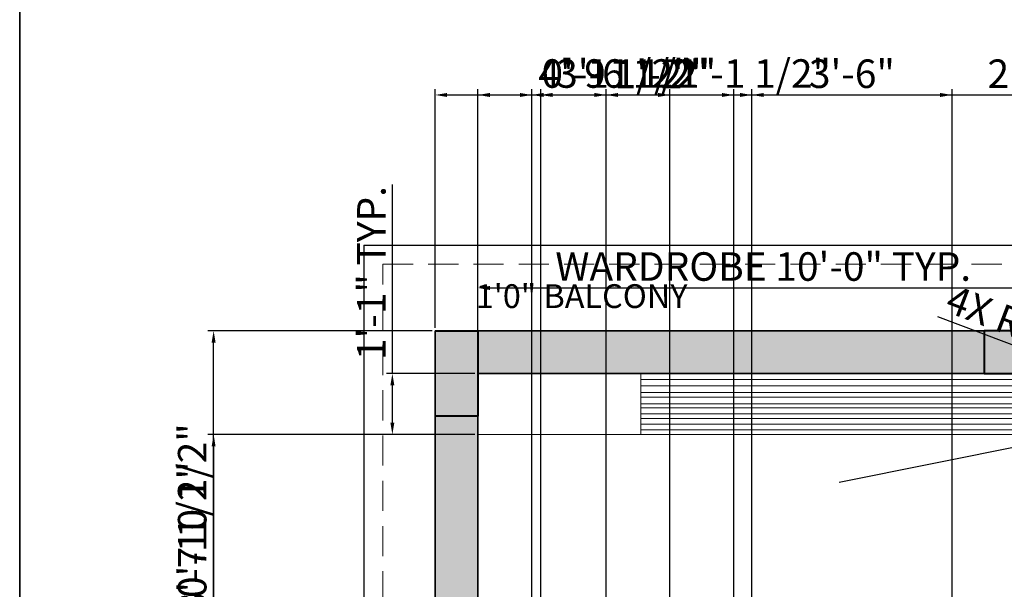
# Model space of a CAD drawing. Units: inches. Extents: x 2656 to 9931, y 1941 to 3068.
# Tile 13 of 46: x 2656 to 2863, y 2569 to 2689. Entities that reach past the tile are written whole.
import ezdxf

# ---------------------------------------------------------------- set-up
doc = ezdxf.new("R2010")
doc.units = ezdxf.units.IN
doc.linetypes.add('DASHED2', pattern=[9.525, 6.35, -3.175])
for name, color, linetype, lineweight in [('A-ANNO-DIMS', 2, 'Continuous', 18), ('A-ANNO-TTLB', 7, 'Continuous', 35), ('A-AREA-IDEN', 7, 'Continuous', 18), ('A-COLS', 7, 'Continuous', 40), ('A-COLS-PATT', 146, 'Continuous', 13), ('A-FLOR-CASE', 32, 'Continuous', 18), ('A-FLOR-OVHD', 252, 'DASHED2', 13), ('A-WALL', 7, 'Continuous', 35), ('A-WALL-PATT', 251, 'Continuous', 13), ('C-PROP', 7, 'Continuous', 25)]:
    doc.layers.add(name, color=color, linetype=linetype, lineweight=lineweight)
doc.styles.get("Standard").update_dxf_attribs({"font": 'arial.ttf'})
doc.dimstyles.new('ISO-25', dxfattribs={"dimtxt": 6, "dimasz": 2.5, "dimexe": 1.25, "dimexo": 0.625, "dimtad": 1, "dimdec": 0, "dimlunit": 3, "dimtxsty": 'Standard', "dimcen": 2.5, "dimadec": 0, "dimazin": 0, "dimtfac": 1, "dimtdec": 0, "dimtmove": 0, "dimatfit": 3, "dimfxl": 1, "dimarcsym": 0})

# ---------------------------------------------------------------- blocks, each defined once
blk = doc.blocks.new('WARDROBE-LONG')
for p, q in [((34.19, 12.8), (34.19, -0.03)), ((34.19, 11.55), (119.96, 11.55)), ((34.19, 10.19), (119.96, 10.19)), ((34.19, 8.82), (119.96, 8.82)), ((34.19, 7.81), (119.96, 7.81)), ((34.19, 6.39), (119.96, 6.39)), ((34.19, 5.58), (119.96, 5.58)), ((34.19, 4.35), (119.96, 4.35)), ((34.19, 3.33), (119.96, 3.33)), ((34.19, 2.12), (119.96, 2.12)), ((34.19, 2.12), (119.96, 2.12)), ((34.19, -0.03), (34.19, 0.97)), ((34.19, 0.97), (119.96, 0.97)), ((-0.04, -0.03), (119.96, -0.03))]:
    blk.add_line(p, q)
blk = doc.blocks.new('*D57')
at = {"layer": 'A-ANNO-DIMS', "color": 0, "lineweight": -2, "transparency": 16777216}
for p, q in [((2752.16, 2615.23), (2752.16, 2633.85)), ((2754.66, 2632.6), (2869.66, 2632.6)), ((2872.16, 2615.23), (2872.16, 2633.85))]:
    blk.add_line(p, q, dxfattribs=at)
at = {"layer": 'A-ANNO-DIMS', "color": 0, "transparency": 16777216}
for points in [[(2754.66, 2633.02), (2754.66, 2632.18), (2752.16, 2632.6)], [(2869.66, 2633.02), (2869.66, 2632.18), (2872.16, 2632.6)]]:
    blk.add_solid(points, dxfattribs=at)
at = {"layer": 'Defpoints', "color": 0, "transparency": 16777216}
for p in [(2872.16, 2632.6), (2752.16, 2614.6), (2872.16, 2614.6)]:
    blk.add_point(p, dxfattribs=at)
at = {"layer": 'A-ANNO-DIMS', "color": 0, "transparency": 16777216, "insert": (2812.16, 2636.33), "char_height": 6, "attachment_point": 5}
blk.add_mtext('WARDROBE 10\'-0" TYP.', dxfattribs=at)
blk = doc.blocks.new('*D58')
at = {"layer": 'A-ANNO-DIMS', "color": 0, "lineweight": -2, "transparency": 16777216}
for p, q in [((2734.16, 2614.6), (2734.16, 2654.36)), ((2751.53, 2614.6), (2732.91, 2614.6)), ((2734.16, 2604.27), (2734.16, 2612.1)), ((2751.53, 2601.77), (2732.91, 2601.77))]:
    blk.add_line(p, q, dxfattribs=at)
at = {"layer": 'A-ANNO-DIMS', "color": 0, "transparency": 16777216}
for points in [[(2733.74, 2612.1), (2734.57, 2612.1), (2734.16, 2614.6)], [(2733.74, 2604.27), (2734.57, 2604.27), (2734.16, 2601.77)]]:
    blk.add_solid(points, dxfattribs=at)
at = {"layer": 'Defpoints', "color": 0, "transparency": 16777216}
for p in [(2734.16, 2614.6), (2752.16, 2614.6), (2752.16, 2601.77)]:
    blk.add_point(p, dxfattribs=at)
at = {"layer": 'A-ANNO-DIMS', "color": 0, "transparency": 16777216, "insert": (2730.52, 2635.73), "char_height": 6, "attachment_point": 5, "rotation": 90}
blk.add_mtext('1\'-1" TYP.', dxfattribs=at)
blk = doc.blocks.new('*D100')
at = {"layer": 'A-ANNO-DIMS', "color": 0, "lineweight": -2, "transparency": 16777216}
for p, q in [((2696.56, 2565.34), (2696.56, 2603.68)), ((2876.03, 2565.34), (2695.31, 2565.34)), ((2696.56, 2557.1), (2696.56, 2562.84)), ((2876.03, 2554.6), (2695.31, 2554.6))]:
    blk.add_line(p, q, dxfattribs=at)
at = {"layer": 'A-ANNO-DIMS', "color": 0, "transparency": 16777216}
for points in [[(2696.14, 2562.84), (2696.97, 2562.84), (2696.56, 2565.34)], [(2696.14, 2557.1), (2696.97, 2557.1), (2696.56, 2554.6)]]:
    blk.add_solid(points, dxfattribs=at)
at = {"layer": 'Defpoints', "color": 0, "transparency": 16777216}
for p in [(2696.56, 2565.34), (2876.66, 2565.34), (2876.66, 2554.6)]:
    blk.add_point(p, dxfattribs=at)
at = {"layer": 'A-ANNO-DIMS', "color": 0, "transparency": 16777216, "insert": (2692.83, 2585.76), "char_height": 6, "attachment_point": 5, "rotation": 90}
blk.add_mtext('0\'-10 1/2"', dxfattribs=at)
blk = doc.blocks.new('*D113')
at = {"layer": 'A-ANNO-DIMS', "color": 0, "lineweight": -2, "transparency": 16777216}
for p, q in [((2752.16, 2300.73), (2752.16, 2674.45)), ((2809.77, 2300.73), (2809.77, 2674.45)), ((2754.66, 2673.2), (2807.27, 2673.2))]:
    blk.add_line(p, q, dxfattribs=at)
at = {"layer": 'A-ANNO-DIMS', "color": 0, "transparency": 16777216}
for points in [[(2754.66, 2673.62), (2754.66, 2672.78), (2752.16, 2673.2)], [(2807.27, 2673.62), (2807.27, 2672.78), (2809.77, 2673.2)]]:
    blk.add_solid(points, dxfattribs=at)
at = {"layer": 'Defpoints', "color": 0, "transparency": 16777216}
for p in [(2809.77, 2673.2), (2752.16, 2300.1), (2809.77, 2300.1)]:
    blk.add_point(p, dxfattribs=at)
at = {"layer": 'A-ANNO-DIMS', "color": 0, "transparency": 16777216, "insert": (2780.96, 2676.93), "char_height": 6, "attachment_point": 5}
blk.add_mtext('4\'-9 1/2"', dxfattribs=at)
blk = doc.blocks.new('*D114')
at = {"layer": 'A-ANNO-DIMS', "color": 0, "lineweight": -2, "transparency": 16777216}
for p, q in [((2809.77, 2300.73), (2809.77, 2674.45)), ((2851.88, 2300.73), (2851.88, 2674.45)), ((2812.27, 2673.2), (2849.38, 2673.2))]:
    blk.add_line(p, q, dxfattribs=at)
at = {"layer": 'A-ANNO-DIMS', "color": 0, "transparency": 16777216}
for points in [[(2812.27, 2673.62), (2812.27, 2672.78), (2809.77, 2673.2)], [(2849.38, 2673.62), (2849.38, 2672.78), (2851.88, 2673.2)]]:
    blk.add_solid(points, dxfattribs=at)
at = {"layer": 'Defpoints', "color": 0, "transparency": 16777216}
for p in [(2851.88, 2673.2), (2809.77, 2300.1), (2851.88, 2300.1)]:
    blk.add_point(p, dxfattribs=at)
at = {"layer": 'A-ANNO-DIMS', "color": 0, "transparency": 16777216, "insert": (2830.82, 2676.89), "char_height": 6, "attachment_point": 5}
blk.add_mtext('3\'-6"', dxfattribs=at)
blk = doc.blocks.new('*D128')
at = {"layer": 'A-ANNO-DIMS', "color": 0, "lineweight": -2, "transparency": 16777216}
for p, q in [((2751.53, 2601.77), (2695.31, 2601.77)), ((2696.56, 2599.27), (2696.56, 2560.87)), ((2776.96, 2558.37), (2695.31, 2558.37))]:
    blk.add_line(p, q, dxfattribs=at)
at = {"layer": 'A-ANNO-DIMS', "color": 0, "transparency": 16777216}
for points in [[(2696.14, 2599.27), (2696.97, 2599.27), (2696.56, 2601.77)], [(2696.14, 2560.87), (2696.97, 2560.87), (2696.56, 2558.37)]]:
    blk.add_solid(points, dxfattribs=at)
at = {"layer": 'Defpoints', "color": 0, "transparency": 16777216}
for p in [(2752.16, 2601.77), (2696.56, 2558.37), (2777.59, 2558.37)]:
    blk.add_point(p, dxfattribs=at)
at = {"layer": 'A-ANNO-DIMS', "color": 0, "transparency": 16777216, "insert": (2692.83, 2580.07), "char_height": 6, "attachment_point": 5, "rotation": 90}
blk.add_mtext('3\'-7 1/2"', dxfattribs=at)
blk = doc.blocks.new('*D129')
at = {"layer": 'A-ANNO-DIMS', "color": 0, "lineweight": -2, "transparency": 16777216}
for p, q in [((2752.16, 2601.15), (2752.16, 2009.27)), ((2777.59, 2557.74), (2777.59, 2009.27)), ((2754.66, 2010.52), (2775.09, 2010.52)), ((2777.59, 2010.52), (2811.37, 2010.52))]:
    blk.add_line(p, q, dxfattribs=at)
at = {"layer": 'A-ANNO-DIMS', "color": 0, "transparency": 16777216}
for points in [[(2754.66, 2010.94), (2754.66, 2010.11), (2752.16, 2010.52)], [(2775.09, 2010.94), (2775.09, 2010.11), (2777.59, 2010.52)]]:
    blk.add_solid(points, dxfattribs=at)
at = {"layer": 'Defpoints', "color": 0, "transparency": 16777216}
for p in [(2752.16, 2601.77), (2777.59, 2558.37), (2777.59, 2010.52)]:
    blk.add_point(p, dxfattribs=at)
at = {"layer": 'A-ANNO-DIMS', "color": 0, "transparency": 16777216, "insert": (2795.73, 2014.25), "char_height": 6, "attachment_point": 5}
blk.add_mtext('2\'-1 1/2"', dxfattribs=at)
blk = doc.blocks.new('*D132')
at = {"layer": 'A-ANNO-DIMS', "color": 0, "lineweight": -2, "transparency": 16777216}
for p, q in [((2763.47, 2366.56), (2763.47, 2674.45)), ((2805.96, 2366.56), (2805.96, 2674.45)), ((2765.97, 2673.2), (2803.46, 2673.2))]:
    blk.add_line(p, q, dxfattribs=at)
at = {"layer": 'A-ANNO-DIMS', "color": 0, "transparency": 16777216}
for points in [[(2765.97, 2673.62), (2765.97, 2672.78), (2763.47, 2673.2)], [(2803.46, 2673.62), (2803.46, 2672.78), (2805.96, 2673.2)]]:
    blk.add_solid(points, dxfattribs=at)
at = {"layer": 'Defpoints', "color": 0, "transparency": 16777216}
for p in [(2805.96, 2673.2), (2763.47, 2365.93), (2805.96, 2365.93)]:
    blk.add_point(p, dxfattribs=at)
at = {"layer": 'A-ANNO-DIMS', "color": 0, "transparency": 16777216, "insert": (2784.72, 2676.93), "char_height": 6, "attachment_point": 5}
blk.add_mtext('3\'-6 1/2"', dxfattribs=at)
blk = doc.blocks.new('*D134')
at = {"layer": 'A-ANNO-DIMS', "color": 0, "lineweight": -2, "transparency": 16777216}
for p, q in [((2752.16, 2300.73), (2752.16, 2674.45)), ((2763.47, 2347.43), (2763.47, 2674.45)), ((2754.66, 2673.2), (2760.97, 2673.2)), ((2763.47, 2673.2), (2801.81, 2673.2))]:
    blk.add_line(p, q, dxfattribs=at)
at = {"layer": 'A-ANNO-DIMS', "color": 0, "transparency": 16777216}
for points in [[(2754.66, 2673.62), (2754.66, 2672.78), (2752.16, 2673.2)], [(2760.97, 2673.62), (2760.97, 2672.78), (2763.47, 2673.2)]]:
    blk.add_solid(points, dxfattribs=at)
at = {"layer": 'Defpoints', "color": 0, "transparency": 16777216}
for p in [(2763.47, 2673.2), (2763.47, 2346.81), (2752.16, 2300.1)]:
    blk.add_point(p, dxfattribs=at)
at = {"layer": 'A-ANNO-DIMS', "color": 0, "transparency": 16777216, "insert": (2783.89, 2676.93), "char_height": 6, "attachment_point": 5}
blk.add_mtext('0\'-11 1/2"', dxfattribs=at)
blk = doc.blocks.new('*D136')
at = {"layer": 'A-ANNO-DIMS', "color": 0, "lineweight": -2, "transparency": 16777216}
for p, q in [((2765.36, 2375.04), (2765.36, 2674.45)), ((2779.14, 2375.04), (2779.14, 2674.45)), ((2767.86, 2673.2), (2776.64, 2673.2)), ((2779.14, 2673.2), (2798.28, 2673.2))]:
    blk.add_line(p, q, dxfattribs=at)
at = {"layer": 'A-ANNO-DIMS', "color": 0, "transparency": 16777216}
for points in [[(2767.86, 2673.62), (2767.86, 2672.78), (2765.36, 2673.2)], [(2776.64, 2673.62), (2776.64, 2672.78), (2779.14, 2673.2)]]:
    blk.add_solid(points, dxfattribs=at)
at = {"layer": 'Defpoints', "color": 0, "transparency": 16777216}
for p in [(2779.14, 2673.2), (2765.36, 2374.42), (2779.14, 2374.42)]:
    blk.add_point(p, dxfattribs=at)
at = {"layer": 'A-ANNO-DIMS', "color": 0, "transparency": 16777216, "insert": (2789.96, 2676.84), "char_height": 6, "attachment_point": 5}
blk.add_mtext('1\'-2"', dxfattribs=at)
blk = doc.blocks.new('*D137')
at = {"layer": 'A-ANNO-DIMS', "color": 0, "lineweight": -2, "transparency": 16777216}
for p, q in [((2779.14, 2375.04), (2779.14, 2674.45)), ((2792.52, 2375.04), (2792.52, 2674.45)), ((2781.64, 2673.2), (2790.02, 2673.2)), ((2792.52, 2673.2), (2825.63, 2673.2))]:
    blk.add_line(p, q, dxfattribs=at)
at = {"layer": 'A-ANNO-DIMS', "color": 0, "transparency": 16777216}
for points in [[(2781.64, 2673.62), (2781.64, 2672.78), (2779.14, 2673.2)], [(2790.02, 2673.62), (2790.02, 2672.78), (2792.52, 2673.2)]]:
    blk.add_solid(points, dxfattribs=at)
at = {"layer": 'Defpoints', "color": 0, "transparency": 16777216}
for p in [(2792.52, 2673.2), (2779.14, 2374.42), (2792.52, 2374.42)]:
    blk.add_point(p, dxfattribs=at)
at = {"layer": 'A-ANNO-DIMS', "color": 0, "transparency": 16777216, "insert": (2810.32, 2676.93), "char_height": 6, "attachment_point": 5}
blk.add_mtext('1\'-1 1/2"', dxfattribs=at)
blk = doc.blocks.new('*D174')
at = {"layer": 'A-ANNO-DIMS', "color": 0, "lineweight": -2, "transparency": 16777216}
for p, q in [((2743.16, 2624.23), (2743.16, 2674.45)), ((2998.16, 2624.23), (2998.16, 2674.45)), ((2745.66, 2673.2), (2995.66, 2673.2))]:
    blk.add_line(p, q, dxfattribs=at)
at = {"layer": 'A-ANNO-DIMS', "color": 0, "transparency": 16777216}
for points in [[(2745.66, 2673.62), (2745.66, 2672.78), (2743.16, 2673.2)], [(2995.66, 2673.62), (2995.66, 2672.78), (2998.16, 2673.2)]]:
    blk.add_solid(points, dxfattribs=at)
at = {"layer": 'Defpoints', "color": 0, "transparency": 16777216}
for p in [(2998.16, 2673.2), (2743.16, 2623.6), (2998.16, 2623.6)]:
    blk.add_point(p, dxfattribs=at)
at = {"layer": 'A-ANNO-DIMS', "color": 0, "transparency": 16777216, "insert": (2870.66, 2676.89), "char_height": 6, "attachment_point": 5}
blk.add_mtext('21\'-3"', dxfattribs=at)
blk = doc.blocks.new('*D175')
at = {"layer": 'A-ANNO-DIMS', "color": 0, "lineweight": -2, "transparency": 16777216}
for p, q in [((2742.53, 2623.6), (2695.31, 2623.6)), ((2696.56, 2169.1), (2696.56, 2621.1)), ((2742.53, 2166.6), (2695.31, 2166.6))]:
    blk.add_line(p, q, dxfattribs=at)
at = {"layer": 'A-ANNO-DIMS', "color": 0, "transparency": 16777216}
for points in [[(2696.14, 2621.1), (2696.97, 2621.1), (2696.56, 2623.6)], [(2696.14, 2169.1), (2696.97, 2169.1), (2696.56, 2166.6)]]:
    blk.add_solid(points, dxfattribs=at)
at = {"layer": 'Defpoints', "color": 0, "transparency": 16777216}
for p in [(2696.56, 2623.6), (2743.16, 2623.6), (2743.16, 2166.6)]:
    blk.add_point(p, dxfattribs=at)
at = {"layer": 'A-ANNO-DIMS', "color": 0, "transparency": 16777216, "insert": (2692.87, 2395.1), "char_height": 6, "attachment_point": 5, "rotation": 90}
blk.add_mtext('38\'-1"', dxfattribs=at)
blk = doc.blocks.new('*D189')
at = {"layer": 'A-ANNO-DIMS', "color": 0, "lineweight": -2, "transparency": 16777216}
for p, q in [((2958.39, 2618.02), (2900.95, 2606.42)), ((2828.14, 2591.72), (2898.5, 2605.92))]:
    blk.add_line(p, q, dxfattribs=at)
at = {"layer": 'A-ANNO-DIMS', "color": 0, "transparency": 16777216}
blk.add_solid([(2900.86, 2606.83), (2901.03, 2606.01), (2898.5, 2605.92)], dxfattribs=at)
at = {"layer": 'Defpoints', "color": 0, "transparency": 16777216}
for p in [(2898.5, 2605.92), (2828.14, 2591.72)]:
    blk.add_point(p, dxfattribs=at)
at = {"layer": 'A-ANNO-DIMS', "color": 0, "transparency": 16777216, "insert": (2939.98, 2618.06), "char_height": 6, "attachment_point": 5, "rotation": 11.4157}
blk.add_mtext('4X R6\'-0"', dxfattribs=at)
blk = doc.blocks.new('*D192')
at = {"layer": 'A-ANNO-DIMS', "color": 0, "lineweight": -2, "transparency": 16777216}
for p, q in [((2848.84, 2626.63), (2897.99, 2608.01)), ((2907.35, 2604.47), (2900.33, 2607.13))]:
    blk.add_line(p, q, dxfattribs=at)
at = {"layer": 'A-ANNO-DIMS', "color": 0, "transparency": 16777216}
blk.add_solid([(2898.14, 2608.4), (2897.84, 2607.62), (2900.33, 2607.13)], dxfattribs=at)
at = {"layer": 'Defpoints', "color": 0, "transparency": 16777216}
for p in [(2900.33, 2607.13), (2907.35, 2604.47)]:
    blk.add_point(p, dxfattribs=at)
at = {"layer": 'A-ANNO-DIMS', "color": 0, "transparency": 16777216, "insert": (2873.57, 2621.25), "char_height": 6, "attachment_point": 5, "rotation": 339.2505}
blk.add_mtext('4X R0\'-7 1/2"', dxfattribs=at)

msp = doc.modelspace()

# ---------------------------------------------------------------- hatches: boundary and pattern name
at = {"layer": 'A-COLS-PATT'}
h = msp.add_hatch(color=256, dxfattribs=at)
h.dxf.hatch_style = 1
h.paths.add_polyline_path([(2752.16, 2623.6), (2743.16, 2623.6), (2743.16, 2605.6), (2752.16, 2605.6)])
h.paths.add_polyline_path([(2876.66, 2623.6), (2858.66, 2623.6), (2858.66, 2614.6), (2876.66, 2614.6)])
h.paths.add_polyline_path([(2998.16, 2623.6), (2989.16, 2623.6), (2989.16, 2614.6), (2989.16, 2605.6), (2998.16, 2605.6)])
h.paths.add_polyline_path([(2998.16, 2444.1), (2989.16, 2444.1), (2989.16, 2426.1), (2998.16, 2426.1)])
h.paths.add_polyline_path([(2876.66, 2444.1), (2867.66, 2444.1), (2867.66, 2426.1), (2876.66, 2426.1)])
h.paths.add_polyline_path([(2752.16, 2444.1), (2743.16, 2444.1), (2743.16, 2426.1), (2752.16, 2426.1)])
h.paths.add_polyline_path([(2752.16, 2300.1), (2743.16, 2300.1), (2743.16, 2282.1), (2752.16, 2282.1)])
h.paths.add_polyline_path([(2876.66, 2300.1), (2867.66, 2300.1), (2867.66, 2282.1), (2876.66, 2282.1)])
h.paths.add_polyline_path([(2998.16, 2300.1), (2989.16, 2300.1), (2989.16, 2282.1), (2998.16, 2282.1)])
h.paths.add_polyline_path([(2998.16, 2184.6), (2989.16, 2184.6), (2989.16, 2166.6), (2998.16, 2166.6)])
h.paths.add_polyline_path([(2876.66, 2175.6), (2858.66, 2175.6), (2858.66, 2166.6), (2876.66, 2166.6)])
h.paths.add_polyline_path([(2752.16, 2184.6), (2743.16, 2184.6), (2743.16, 2166.6), (2752.16, 2166.6)])
at = {"layer": 'A-WALL-PATT'}
h = msp.add_hatch(color=256, dxfattribs=at)
h.dxf.hatch_style = 1
h.paths.add_polyline_path([(2858.66, 2623.6), (2752.16, 2623.6), (2752.16, 2614.6), (2858.66, 2614.6)])
h.paths.add_polyline_path([(2893.09, 2623.6), (2876.66, 2623.6), (2876.66, 2614.6), (2893.09, 2614.6), (2893.09, 2619.1)])
h.paths.add_polyline_path([(2946.51, 2623.6), (2917.09, 2623.6), (2917.09, 2614.6), (2946.51, 2614.6), (2946.51, 2619.1)])
h.paths.add_polyline_path([(2989.16, 2623.6), (2970.51, 2623.6), (2970.51, 2614.6), (2989.16, 2614.6)])
h.paths.add_polyline_path([(2998.16, 2605.6), (2989.16, 2605.6), (2989.16, 2523.88), (2998.16, 2523.88)])
h.paths.add_polyline_path([(2935.16, 2614.6), (2930.66, 2614.6), (2930.66, 2554.6), (2876.66, 2554.6), (2876.66, 2565.34), (2872.16, 2565.34), (2872.16, 2444.1), (2876.66, 2444.1), (2876.66, 2550.1), (2946.47, 2550.1), (2946.47, 2554.6), (2935.16, 2554.6)])
h.paths.add_polyline_path([(2989.16, 2554.6), (2982.11, 2554.6), (2976.57, 2554.6), (2976.57, 2550.1), (2982.11, 2550.1), (2989.16, 2550.1)])
h.paths.add_polyline_path([(2876.66, 2614.6), (2872.16, 2614.6), (2872.16, 2595), (2876.66, 2595)], flags=0)
h.paths.add_polyline_path([(2752.16, 2605.6), (2743.16, 2605.6), (2743.16, 2544.03), (2752.16, 2544.03)])
h.paths.add_polyline_path([(2752.16, 2426.1), (2743.16, 2426.1), (2743.16, 2300.1), (2752.16, 2300.1)])
h.paths.add_polyline_path([(2821.13, 2430.6), (2752.16, 2430.6), (2752.16, 2426.1), (2821.13, 2426.1)])
h.paths.add_polyline_path([(2867.66, 2430.6), (2862.88, 2430.6), (2862.88, 2426.1), (2867.66, 2426.1)])
h.paths.add_polyline_path([(2752.16, 2484.03), (2747.66, 2484.03), (2743.16, 2484.03), (2743.16, 2444.1), (2752.16, 2444.1)])
h.paths.add_polyline_path([(2998.16, 2426.1), (2989.16, 2426.1), (2989.16, 2390.1), (2872.16, 2390.1), (2872.16, 2385.6), (2876.66, 2385.6), (2989.16, 2385.6), (2989.16, 2365.04), (2998.16, 2365.04)])
h.paths.add_polyline_path([(2998.16, 2463.88), (2993.66, 2463.88), (2989.16, 2463.88), (2989.16, 2444.1), (2998.16, 2444.1)])
h.paths.add_polyline_path([(2998.16, 2319.88), (2989.16, 2319.88), (2989.16, 2300.1), (2998.16, 2300.1)])
h.paths.add_polyline_path([(2998.16, 2282.1), (2989.16, 2282.1), (2989.16, 2253.6), (2982.06, 2253.6), (2982.06, 2249.1), (2989.16, 2249.1), (2998.16, 2249.1)])
h.paths.add_polyline_path([(2931.54, 2253.6), (2923.8, 2253.6), (2923.8, 2249.1), (2931.54, 2249.1)])
h.paths.add_polyline_path([(2876.66, 2282.1), (2872.16, 2282.1), (2872.16, 2184.6), (2872.16, 2175.6), (2876.66, 2175.6), (2876.66, 2249.1), (2888.32, 2249.1), (2888.32, 2251.35), (2888.32, 2253.6), (2876.66, 2253.6)])
h.paths.add_polyline_path([(2858.66, 2175.6), (2841.42, 2175.6), (2841.42, 2166.6), (2858.66, 2166.6)])
h.paths.add_polyline_path([(2785.06, 2171.1), (2785.06, 2175.6), (2752.16, 2175.6), (2752.16, 2166.6), (2785.06, 2166.6)])
h.paths.add_polyline_path([(2752.16, 2282.1), (2743.16, 2282.1), (2743.16, 2184.6), (2752.16, 2184.6)])
h.paths.add_polyline_path([(2809.77, 2300.1), (2752.16, 2300.1), (2752.16, 2295.6), (2809.77, 2295.6)])
h.paths.add_polyline_path([(2867.66, 2300.1), (2851.88, 2300.1), (2851.88, 2295.6), (2867.66, 2295.6)])

# ---------------------------------------------------------------- linework, layer by layer
at = {"layer": 'A-ANNO-TTLB'}
msp.add_lwpolyline([(2655.77, 3067.84), (3515.43, 3067.84), (3515.43, 1940.89), (2655.77, 1940.89)], close=True, dxfattribs=at)
at = {"layer": 'A-COLS'}
for p, q in [((2743.16, 2623.6), (2752.16, 2623.6)), ((2752.16, 2623.6), (2752.16, 2605.6)), ((2876.66, 2623.6), (2858.66, 2623.6)), ((2858.66, 2623.6), (2858.66, 2614.6)), ((2858.66, 2614.6), (2876.66, 2614.6)), ((2752.16, 2605.6), (2743.16, 2605.6))]:
    msp.add_line(p, q, dxfattribs=at)
at = {"layer": 'A-FLOR-OVHD'}
for p, q in [((2732.16, 2166.6), (2732.16, 2637.6)), ((2732.16, 2637.6), (3024.16, 2637.6))]:
    msp.add_line(p, q, dxfattribs=at)
at = {"layer": 'A-WALL'}
for p, q in [((2743.16, 2623.6), (2743.16, 2166.6)), ((2743.16, 2623.6), (2998.16, 2623.6)), ((2752.16, 2614.6), (2752.16, 2166.6)), ((2752.16, 2614.6), (2989.16, 2614.6))]:
    msp.add_line(p, q, dxfattribs=at)
at = {"layer": 'C-PROP'}
for q in [(2728.16, 2086.1), (3028.16, 2641.6)]:
    msp.add_line((2728.16, 2641.6), q, dxfattribs=at)

# ---------------------------------------------------------------- block references
at = {"layer": 'A-FLOR-CASE'}
msp.add_blockref('WARDROBE-LONG', (2752.2, 2601.8), dxfattribs=at)

# ---------------------------------------------------------------- texts
at = {"layer": 'A-AREA-IDEN', "insert": (2751.71, 2633.38), "char_height": 5, "attachment_point": 1}
msp.add_mtext_dynamic_manual_height_columns('1\'0" BALCONY', width=95.951, gutter_width=12.5, heights=[0], dxfattribs=at)

# ---------------------------------------------------------------- dimensions: what is measured, and where the dimension line sits
at = {"layer": 'A-ANNO-DIMS'}
for base, p1, p2, picture, middle in [((2809.77, 2673.2), (2752.16, 2300.1), (2809.77, 2300.1), '*D113', (2780.96, 2676.93)), ((2763.47, 2673.2), (2752.16, 2300.1), (2763.47, 2346.81), '*D134', (2783.89, 2676.93)), ((2805.96, 2673.2), (2763.47, 2365.93), (2805.96, 2365.93), '*D132', (2784.72, 2676.93)), ((2792.52, 2673.2), (2779.14, 2374.42), (2792.52, 2374.42), '*D137', (2810.32, 2676.93)), ((2998.16, 2673.2), (2743.16, 2623.6), (2998.16, 2623.6), '*D174', (2870.66, 2676.89)), ((2779.14, 2673.2), (2765.36, 2374.42), (2779.14, 2374.42), '*D136', (2789.96, 2676.84)), ((2851.88, 2673.2), (2809.77, 2300.1), (2851.88, 2300.1), '*D114', (2830.82, 2676.89)), ((2777.59, 2010.52), (2752.16, 2601.77), (2777.59, 2558.37), '*D129', (2795.73, 2014.25))]:
    dim = msp.add_linear_dim(base=base, p1=p1, p2=p2, dimstyle='ISO-25', override={"dimdec": 1, "dimlfac": 1, "dimrnd": 0, "dimzin": 1, "dimdsep": 46, "dimlunit": 4, "dimfrac": 2}, dxfattribs=at)
    dim.commit()
    dim.dimension.update_dxf_attribs({"geometry": picture, "text_midpoint": middle})
dim = msp.add_linear_dim(base=(2734.16, 2614.6), p1=(2752.16, 2601.77), p2=(2752.16, 2614.6), angle=90, text='<> TYP.', dimstyle='ISO-25', override={"dimdec": 1, "dimlfac": 1, "dimrnd": 0, "dimzin": 1, "dimdsep": 46, "dimlunit": 4, "dimfrac": 2}, dxfattribs=at)
dim.commit()
dim.dimension.update_dxf_attribs({"geometry": '*D58', "text_midpoint": (2730.52, 2635.73)})
dim = msp.add_linear_dim(base=(2872.16, 2632.6), p1=(2752.16, 2614.6), p2=(2872.16, 2614.6), text='WARDROBE <> TYP.', dimstyle='ISO-25', override={"dimdec": 1, "dimlfac": 1, "dimrnd": 0, "dimzin": 1, "dimdsep": 46, "dimlunit": 4, "dimfrac": 2}, dxfattribs=at)
dim.commit()
dim.dimension.update_dxf_attribs({"geometry": '*D57', "text_midpoint": (2812.16, 2636.33)})
dim = msp.add_radius_dim(center=(2907.35, 2604.47), mpoint=(2900.33, 2607.13), text='4X <>', dimstyle='ISO-25', override={"dimdec": 1, "dimlfac": 1, "dimrnd": 0, "dimzin": 1, "dimdsep": 46, "dimlunit": 4, "dimfrac": 2}, dxfattribs=at)
dim.commit()
dim.dimension.update_dxf_attribs({"geometry": '*D192', "text_midpoint": (2873.57, 2621.25)})
dim = msp.add_radius_dim(center=(2828.14, 2591.72), mpoint=(2898.5, 2605.92), text='4X <>', dimstyle='ISO-25', override={"dimdec": 1, "dimlfac": 1, "dimrnd": 0, "dimzin": 1, "dimdsep": 46, "dimlunit": 4, "dimfrac": 2}, dxfattribs=at)
dim.commit()
dim.dimension.update_dxf_attribs({"geometry": '*D189', "text_midpoint": (2940.71, 2614.45), "dimtype": 164})
for base, p1, p2, picture, middle in [((2696.56, 2623.6), (2743.16, 2166.6), (2743.16, 2623.6), '*D175', (2692.87, 2395.1)), ((2696.56, 2565.34), (2876.66, 2554.6), (2876.66, 2565.34), '*D100', (2692.83, 2585.76)), ((2696.56, 2558.37), (2752.16, 2601.77), (2777.59, 2558.37), '*D128', (2692.83, 2580.07))]:
    dim = msp.add_linear_dim(base=base, p1=p1, p2=p2, angle=90, dimstyle='ISO-25', override={"dimdec": 1, "dimlfac": 1, "dimrnd": 0, "dimzin": 1, "dimdsep": 46, "dimlunit": 4, "dimfrac": 2}, dxfattribs=at)
    dim.commit()
    dim.dimension.update_dxf_attribs({"geometry": picture, "text_midpoint": middle})

doc.saveas('drawing.dxf')
